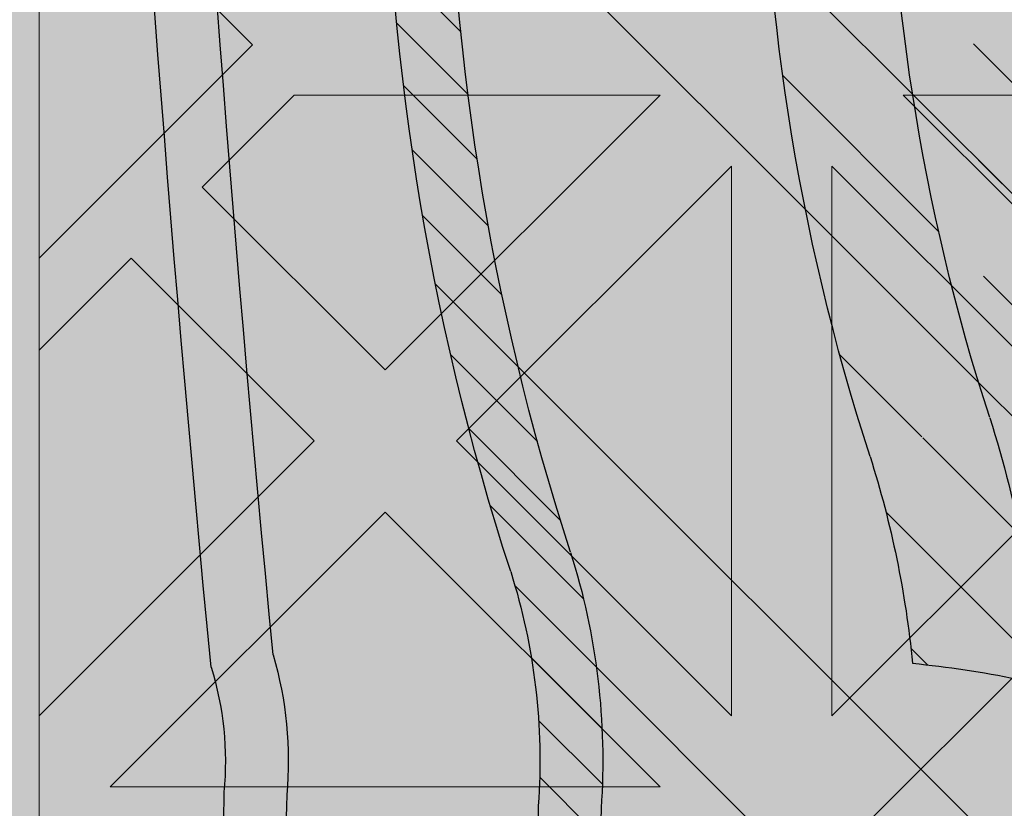
# Model space of a CAD drawing. Units: inches. Extents: x 844 to 2234, y 346 to 1084.
# Tile 28 of 93: x 1252.862 to 1255.358, y 689.183 to 691.183. Entities that reach past the tile are written whole.
import ezdxf

# ---------------------------------------------------------------- set-up
doc = ezdxf.new("R2010")
doc.units = ezdxf.units.IN
doc.header["$MEASUREMENT"] = 0
doc.layers.add('furniture', color=8, linetype='Continuous', lineweight=18)
doc.layers.add('RA-AP-01$0$INT', color=35, linetype='Continuous', lineweight=5)
doc.layers.add('RA-AP-01$0$FURN', color=3, linetype='Continuous')
doc.layers.add('RA-AP-01$0$WOOD', color=64, linetype='Continuous')

# ---------------------------------------------------------------- blocks, each defined once
blk = doc.blocks.new('A$C18D01794')
at = {"layer": 'RA-AP-01$0$INT'}
blk.add_hatch(color=256, dxfattribs=at).paths.add_polyline_path([(4.505206456958071, -6.306712009588038), (5.305206456958072, -6.306712009588038), (5.305206456958072, -7.106712009588038), (5.255206456951893, -7.10671200958804), (5.25520645694868, -6.356712009605972), (4.555206456959269, -6.356712009587461), (4.555206456956052, -7.106712009588038), (4.505206456958073, -7.106712009588038)])
h = blk.add_hatch(color=256, dxfattribs=at)
h.paths.add_polyline_path([(4.585917135068449, -6.356712009588271), (4.555206456959269, -6.35671200958746), (4.555206456959137, -6.387422687716308), (4.874495778835233, -6.706712009592356), (4.90520645695423, -6.676001331474049)])
h.paths.add_polyline_path([(5.255206456948813, -6.387422687716306), (5.255206456948682, -6.356712009605972), (5.224495778822613, -6.356712009605161), (4.905206456953498, -6.676001331474273), (4.935917135072151, -6.706712009592924)])
h.paths.add_polyline_path([(4.935917135072559, -6.706712009592068), (4.905206456953564, -6.737422687710376), (5.255206456951813, -7.087422687708613), (5.255206456951549, -7.026001331471008)])
h.paths.add_polyline_path([(4.555206456956399, -7.026001331471013), (4.555206456956134, -7.087422687708616), (4.905206456953821, -6.737422687710943), (4.874495778835166, -6.70671200959229)])
h = blk.add_hatch(color=256, dxfattribs=at)
h.paths.add_polyline_path([(4.585917135068448, -6.356712009588273), (4.614201406330596, -6.356712009589021), (4.668846067270487, -6.411356670531338), (4.723490728212344, -6.356712009591912), (4.771774999457151, -6.35671200959319), (4.826419660396886, -6.411356670535356), (4.862780050090322, -6.374996280843536), (4.844495778842715, -6.356712009595112), (4.862780050090411, -6.356712009595595), (4.905206456960182, -6.399138416468211), (4.947632863832445, -6.356712009597838), (4.965917135079675, -6.356712009598322), (4.947632863831759, -6.374996280845421), (4.983993253523576, -6.411356670538857), (5.038637914464627, -6.356712009600247), (5.08692218571208, -6.356712009601523), (5.141566846649976, -6.411356670541852), (5.196211507589851, -6.356712009604411), (5.224495778822615, -6.356712009605161), (4.905206456953975, -6.676001331473793)])
h.paths.add_polyline_path([(4.895206456956031, -6.637717060225675), (4.895206456958921, -6.528427738347902), (4.840561796018589, -6.583072399285802)], flags=16)
h.paths.add_polyline_path([(4.915206456955638, -6.637717060226121), (4.969851117895509, -6.583072399288678), (4.915206456957609, -6.528427738348344)], flags=16)
h.paths.add_polyline_path([(4.826419660395175, -6.568930263661755), (4.881064321335613, -6.514285602723745), (4.771774999456703, -6.514285602720857)], flags=16)
h.paths.add_polyline_path([(4.983993253519558, -6.568930263665262), (5.038637914460456, -6.514285602726792), (4.929348592581548, -6.514285602724816)], flags=16)
h.paths.add_polyline_path([(4.881064321336025, -6.494285602723742), (4.826419660397532, -6.439640941782821), (4.771774999457062, -6.494285602720859)], flags=16)
h.paths.add_polyline_path([(4.929348592582019, -6.494285602724817), (5.038637914460982, -6.494285602726792), (4.983993253522945, -6.439640941786327)], flags=16)
h.paths.add_polyline_path([(4.895206456960191, -6.480143467100443), (4.895206456962115, -6.407422687715913), (4.876922185715016, -6.389138416467584), (4.840561796021581, -6.425498806159401)], flags=16)
h.paths.add_polyline_path([(4.915206456958487, -6.480143467100889), (4.969851117899527, -6.425498806162279), (4.933490728206909, -6.389138416468043), (4.9152064569598, -6.40742268771434)], flags=16)
h.paths.add_polyline_path([(4.757632863832376, -6.480143467096812), (4.812277524772842, -6.425498806158772), (4.757632863834348, -6.370854145217844)], flags=16)
h.paths.add_polyline_path([(4.737632863832376, -6.480143467096286), (4.737632863834348, -6.370854145217375), (4.682988202893906, -6.425498806155385)], flags=16)
h.paths.add_polyline_path([(5.05278005008503, -6.480143467103376), (5.052780050087917, -6.370854145224413), (4.998135389146995, -6.425498806162908)], flags=16)
h.paths.add_polyline_path([(5.072780050085024, -6.480143467103744), (5.127424711025931, -6.42549880616527), (5.072780050087916, -6.370854145224832)], flags=16)
h.paths.add_polyline_path([(4.935917135072783, -6.706712009592292), (5.255206456948811, -6.387422687716309), (5.255206456948932, -6.415706958964177), (5.200561796010279, -6.470351619902839), (5.255206456949403, -6.524996280841948), (5.25520645694961, -6.5732805520894), (5.200561796009787, -6.627925213029239), (5.236922185702417, -6.664285602721864), (5.255206456949919, -6.646001331474357), (5.255206456949998, -6.664285602721898), (5.212780050078687, -6.706712009592262), (5.25520645695036, -6.749138416463932), (5.255206456950438, -6.767422687711313), (5.236922185702424, -6.749138416463297), (5.200561796009796, -6.785498806155928), (5.255206456950753, -6.840143467096874), (5.25520645695096, -6.888427738341682), (5.200561796010322, -6.943072399282328), (5.255206456951428, -6.997717060223427), (5.255206456951547, -7.026001331471006)])
h.paths.add_polyline_path([(5.042988202883395, -6.785498806155427), (5.097632863823085, -6.840143467095101), (5.097632863822622, -6.730854145216193)], flags=16)
h.paths.add_polyline_path([(5.028846067259663, -6.771356670531693), (5.083490728198774, -6.716712009592573), (4.974201406321001, -6.716712009593042)], flags=16)
h.paths.add_polyline_path([(5.117632863823087, -6.840143467095186), (5.172277524762331, -6.785498806155926), (5.11763286382262, -6.730854145216225)], flags=16)
h.paths.add_polyline_path([(5.08349072819877, -6.696712009593886), (5.028846067259652, -6.642067348654775), (4.974201406320998, -6.696712009593438)], flags=16)
h.paths.add_polyline_path([(5.131774999446817, -6.854285602718917), (5.186419660386065, -6.799640941779662), (5.241064321325782, -6.854285602719365)], flags=17)
h.paths.add_polyline_path([(5.131774999446228, -6.716712009592374), (5.186419660386065, -6.771356670532194), (5.222780050079488, -6.734996280838764), (5.204495778832781, -6.716712009592063)], flags=16)
h.paths.add_polyline_path([(5.097632863822613, -6.682569873970264), (5.097632863823061, -6.573280552091354), (5.042988202883383, -6.627925213031044)], flags=16)
h.paths.add_polyline_path([(5.131774999446899, -6.874285602718915), (5.241064321325809, -6.874285602719364), (5.186419660386591, -6.928930263658598)], flags=17)
h.paths.add_polyline_path([(5.131774999446226, -6.696712009594078), (5.204495778830767, -6.696712009594374), (5.22278005007868, -6.67842773834687), (5.186419660386049, -6.642067348654249)], flags=16)
h.paths.add_polyline_path([(5.11763286382262, -6.682569873970225), (5.17227752476232, -6.627925213030515), (5.117632863823064, -6.573280552091267)], flags=16)
h.paths.add_polyline_path([(5.186419660386069, -6.613783077405491), (5.241064321325754, -6.559138416465795), (5.131774999446791, -6.559138416466263)], flags=16)
h.paths.add_polyline_path([(5.131774999446872, -6.539138416466263), (5.24106432132578, -6.539138416465794), (5.186419660386554, -6.484493755526573)], flags=16)
h.paths.add_polyline_path([(5.255206456951811, -7.08742268770861), (5.255206456951895, -7.106712009588038), (4.555206456956052, -7.106712009588038), (4.555206456956136, -7.087422687708617), (4.905206456953973, -6.737422687710788)])
h.paths.add_polyline_path([(4.983993253513404, -6.8444937555241), (4.92934859257295, -6.899138416462108), (5.03863791445186, -6.899138416465014)], flags=16)
h.paths.add_polyline_path([(4.969851117889988, -6.83035161990006), (4.915206456952556, -6.775706958960171), (4.915206456949648, -6.884996280837944)], flags=16)
h.paths.add_polyline_path([(4.929348592572535, -6.919138416462105), (4.983993253511019, -6.973783077403037), (5.038637914451496, -6.919138416465012)], flags=16)
h.paths.add_polyline_path([(5.052780050074912, -6.93328055208906), (4.998135389134438, -6.987925213027088), (5.052780050072919, -7.042569873968025)], flags=16)
h.paths.add_polyline_path([(5.07278005007491, -6.933280552089588), (5.072780050072918, -7.042569873968497), (5.127424711013374, -6.987925213030498)], flags=16)
h.paths.add_polyline_path([(4.89520645695295, -6.775706958959721), (4.840561796013067, -6.830351619897157), (4.895206456950961, -6.884996280837494)], flags=16)
h.paths.add_polyline_path([(4.915206456948365, -6.933280552085403), (4.915206456946434, -7.006001331471951), (4.933490728192729, -7.024285602719066), (4.969851117886972, -6.987925213026453)], flags=16)
h.paths.add_polyline_path([(4.881064321327021, -6.899138416461022), (4.82641966038902, -6.84449375552057), (4.771774999448108, -6.899138416459029)], flags=16)
h.paths.add_polyline_path([(4.895206456950073, -6.933280552084951), (4.840561796009022, -6.987925213023558), (4.876922185700835, -7.024285602716997), (4.895206456948749, -7.006001331469487)], flags=16)
h.paths.add_polyline_path([(4.983993253510392, -7.0020673486505), (4.947632863816944, -7.038427738342319), (4.965917135064043, -7.05671200959023), (5.038637914448995, -7.056712009591555)], flags=16)
h.paths.add_polyline_path([(4.881064321326543, -6.91913841646102), (4.771774999447578, -6.919138416459031), (4.826419660385607, -6.973783077399508)], flags=16)
h.paths.add_polyline_path([(4.905206456946447, -7.014285602717636), (4.862780050074785, -7.056712009588352), (4.947632863816685, -7.056712009589775)], flags=16)
h.paths.add_polyline_path([(5.14156684663679, -7.002067348654549), (5.086922185696452, -7.056712009592438), (5.196211507574223, -7.056712009594425)], flags=16)
h.paths.add_polyline_path([(4.8264196603837, -7.002067348646972), (4.771774999442643, -7.056712009585575), (4.8444957788276, -7.056712009587508), (4.862780050075511, -7.038427738340416)], flags=16)
h.paths.add_polyline_path([(4.812277524760289, -6.98792521302292), (4.757632863822258, -6.933280552082447), (4.757632863819352, -7.042569873961408)], flags=16)
h.paths.add_polyline_path([(4.73763286382226, -6.933280552082079), (4.682988202881349, -6.987925213020536), (4.737632863819352, -7.04256987396099)], flags=16)
h.paths.add_polyline_path([(4.723490728195188, -7.056712009584289), (4.668846067257299, -7.002067348643949), (4.614201406317417, -7.056712009581383)], flags=16)
h.paths.add_polyline_path([(4.597632863829262, -6.706712009592262), (4.555206456957951, -6.664285602721896), (4.555206456958029, -6.646001331474357), (4.573490728205535, -6.664285602721864), (4.609851117898167, -6.627925213029238), (4.555206456958338, -6.573280552089402), (4.555206456958546, -6.524996280841952), (4.60985111789767, -6.470351619902839), (4.555206456959015, -6.415706958964177), (4.555206456959138, -6.387422687716309), (4.874495778835167, -6.70671200959229), (4.5552064569564, -7.026001331471015), (4.555206456956523, -6.997717060223433), (4.609851117897629, -6.94307239928233), (4.555206456956988, -6.888427738341681), (4.555206456957198, -6.840143467096881), (4.609851117898153, -6.78549880615593), (4.573490728205528, -6.749138416463297), (4.555206456957507, -6.76742268771132), (4.555206456957585, -6.749138416463933)])
h.paths.add_polyline_path([(4.712780050085332, -6.730854145216195), (4.712780050084863, -6.840143467095105), (4.767424711024555, -6.785498806155427)], flags=16)
h.paths.add_polyline_path([(4.726922185709173, -6.716712009592573), (4.781566846648288, -6.771356670531693), (4.836211507586949, -6.716712009593043)], flags=16)
h.paths.add_polyline_path([(4.692780050085327, -6.730854145216225), (4.638135389145619, -6.785498806155928), (4.692780050084865, -6.840143467095185)], flags=16)
h.paths.add_polyline_path([(4.726922185709182, -6.696712009593886), (4.836211507586949, -6.696712009593436), (4.7815668466483, -6.642067348654773)], flags=16)
h.paths.add_polyline_path([(4.678637914461726, -6.71671200959237), (4.605917135075169, -6.716712009592063), (4.587632863828464, -6.734996280838766), (4.623993253521887, -6.771356670532195)], flags=16)
h.paths.add_polyline_path([(4.712780050085336, -6.68256987397026), (4.767424711024568, -6.627925213031042), (4.71278005008489, -6.573280552091352)], flags=16)
h.paths.add_polyline_path([(4.678637914461726, -6.696712009594076), (4.623993253521899, -6.642067348654247), (4.587632863829271, -6.67842773834687), (4.605917135077185, -6.696712009594376)], flags=16)
h.paths.add_polyline_path([(4.692780050085336, -6.682569873970228), (4.692780050084889, -6.573280552091267), (4.638135389145632, -6.627925213030515)], flags=16)
h.paths.add_polyline_path([(4.623993253521885, -6.799640941779662), (4.678637914461131, -6.854285602718915), (4.56934859258217, -6.854285602719365)], flags=17)
h.paths.add_polyline_path([(4.623993253521901, -6.613783077405509), (4.678637914461158, -6.559138416466263), (4.569348592582195, -6.559138416465795)], flags=16)
h.paths.add_polyline_path([(4.678637914461051, -6.874285602718915), (4.623993253521361, -6.928930263658598), (4.569348592582143, -6.874285602719364)], flags=17)
h.paths.add_polyline_path([(4.678637914461076, -6.539138416466263), (4.623993253521399, -6.484493755526573), (4.569348592582167, -6.539138416465796)], flags=16)
h = blk.add_hatch(color=256, dxfattribs=at)
h.paths.add_polyline_path([(5.028846067259997, -6.642067348655121), (4.974201406321342, -6.696712009593783), (5.083490728199115, -6.69671200959423)])
h.paths.add_polyline_path([(4.974201406321344, -6.716712009593388), (5.028846067260004, -6.771356670532039), (5.083490728199117, -6.716712009592919)])
h.paths.add_polyline_path([(5.042988202883738, -6.785498806155768), (5.097632863823428, -6.840143467095449), (5.097632863822963, -6.73085414521654)])
h.paths.add_polyline_path([(5.117632863822961, -6.730854145216568), (5.117632863823428, -6.840143467095531), (5.172277524762674, -6.785498806156272)])
h.paths.add_polyline_path([(5.131774999446572, -6.716712009592718), (5.186419660386406, -6.77135667053254), (5.222780050079831, -6.734996280839116), (5.204495778833122, -6.716712009592409)])
h.paths.add_polyline_path([(5.236922185702764, -6.749138416463644), (5.200561796010139, -6.785498806156274), (5.255206456949971, -6.840143467096101), (5.255206456950271, -6.76742268771115)])
h.paths.add_polyline_path([(5.186419660386412, -6.799640941780006), (5.131774999447164, -6.854285602719262), (5.241064321326123, -6.854285602719711)])
h.paths.add_polyline_path([(5.131774999447238, -6.874285602719261), (5.186419660386934, -6.928930263658944), (5.241064321326153, -6.874285602719709)])
h.paths.add_polyline_path([(5.200561796010663, -6.943072399282675), (5.255206456949324, -6.997717060221329), (5.255206456949777, -6.888427738343558)])
h.paths.add_polyline_path([(5.21278005007903, -6.706712009592607), (5.255206456950223, -6.749138416463798), (5.255206456950696, -6.664285602721891)])
h.paths.add_polyline_path([(5.13177499944657, -6.696712009594424), (5.204495778831106, -6.696712009594723), (5.222780050079024, -6.678427738347219), (5.186419660386397, -6.642067348654592)])
h.paths.add_polyline_path([(5.117632863823405, -6.573280552091611), (5.117632863822955, -6.682569873970578), (5.172277524762665, -6.627925213030859)])
h.paths.add_polyline_path([(5.042988202883727, -6.627925213031387), (5.097632863822957, -6.682569873970603), (5.097632863823407, -6.573280552091697)])
h.paths.add_polyline_path([(5.131774999447135, -6.559138416466609), (5.186419660386394, -6.613783077405857), (5.241064321326097, -6.559138416466144)])
h.paths.add_polyline_path([(5.200561796010128, -6.627925213029584), (5.236922185702758, -6.664285602722211), (5.255206456950264, -6.646001331474705), (5.255206456949948, -6.573280552089752)])
h.paths.add_polyline_path([(5.186419660386895, -6.484493755526919), (5.131774999447213, -6.539138416466609), (5.241064321326127, -6.539138416466142)])
h.paths.add_polyline_path([(5.200561796010624, -6.470351619903183), (5.255206456949745, -6.524996280842298), (5.255206456949276, -6.415706958964523)])
for p, q in [((5.255206456951895, -7.106712009588038), (5.255206456948681, -6.356712009605972)), ((4.935917135072783, -6.706712009592292), (5.255206456948813, -6.387422687716307)), ((5.131774999446792, -6.559138416466263), (5.241064321325755, -6.559138416465795)), ((5.131774999446792, -6.559138416466263), (5.186419660386049, -6.613783077405509)), ((5.241064321325755, -6.559138416465795), (5.186419660386049, -6.613783077405509)), ((5.042988202883385, -6.627925213031041), (5.097632863823062, -6.573280552091352)), ((5.097632863823062, -6.573280552091352), (5.097632863822615, -6.682569873970262)), ((5.117632863823062, -6.573280552091267), (5.172277524762319, -6.627925213030515)), ((5.117632863823062, -6.573280552091267), (5.117632863822614, -6.68256987397023)), ((5.255206456949605, -6.573280552089405), (5.200561796009783, -6.627925213029239)), ((5.255206456949918, -6.646001331474357), (5.255206456949605, -6.573280552089405)), ((5.097632863822615, -6.682569873970262), (5.042988202883383, -6.627925213031042)), ((5.117632863822614, -6.68256987397023), (5.172277524762319, -6.627925213030515)), ((5.200561796009783, -6.627925213029238), (5.236922185702415, -6.664285602721863)), ((5.083490728198769, -6.696712009593882), (5.028846067259652, -6.642067348654775)), ((5.131774999446228, -6.696712009594078), (5.186419660386053, -6.642067348654247)), ((5.186419660386051, -6.642067348654247), (5.222780050078681, -6.67842773834687)), ((5.255206456949919, -6.646001331474357), (5.236922185702415, -6.664285602721864)), ((5.212780050078687, -6.706712009592262), (5.255206456950353, -6.664285602721543)), ((5.25520645694988, -6.74913841646345), (5.255206456950353, -6.664285602721543)), ((5.204495778833082, -6.69671200959206), (5.222780050078681, -6.67842773834687)), ((5.08349072819877, -6.696712009593886), (4.974201406320999, -6.696712009593436)), ((5.204495778831179, -6.696712009594376), (5.131774999446228, -6.696712009594078)), ((5.212780050078687, -6.706712009592262), (5.25520645694988, -6.74913841646345))]:
    blk.add_line(p, q, dxfattribs=at)
blk = doc.blocks.new('A$C32926AE1')
at = {"layer": 'RA-AP-01$0$FURN'}
h = blk.add_hatch(dxfattribs=at)
h.set_pattern_fill('ANSI31', color=256, scale=0.1, style=0)
h.set_pattern_definition([(45, (0, 0), (-0.0088388347648318, 0.0088388347648318), [])])
edge = h.paths.add_edge_path(flags=16)
edge.add_arc((4.904771284329206, 4.246793130718756), 0.2603971832811541, 75.22398030683196, 104.7760196931204)
edge.add_arc((4.904771284329206, 4.246793130718756), 0.2603971832811541, 75.223980306832, 104.77601969312039, ccw=False)
edge = h.paths.add_edge_path(flags=16)
edge.add_arc((4.904771284329206, 4.067062675376612), 0.2603971832811541, 255.2239803068796, 284.776019693168)
edge.add_arc((4.904771284329206, 4.067062675376612), 0.2603971832811541, 255.22398030687958, 284.77601969316805, ccw=False)
edge = h.paths.add_edge_path(flags=0)
edge.add_arc((4.904771284329206, 4.067062675376612), 0.2603971832811541, 255.2239803068796, 284.776019693168)
edge.add_arc((4.904771284329206, 4.067062675376612), 0.2603971832811541, 255.22398030687958, 284.77601969316805, ccw=False)
edge = h.paths.add_edge_path(flags=0)
edge.add_arc((4.904771284329206, 4.067062675376612), 0.2603971832811541, 255.2239803068796, 284.776019693168)
edge.add_arc((4.904771284329206, 4.067062675376612), 0.2603971832811541, 255.22398030687958, 284.77601969316805, ccw=False)
edge = h.paths.add_edge_path()
edge.add_arc((4.604388392048174, 4.588829985554312), 0.1599999999999918, 342.3781640246255, 354.4317409793762)
edge.add_arc((5.090145208887507, 4.43216705527679), 0.3503971832811637, 162.0091218307731, 180.3186872093483)
edge.add_arc((5.205154176610243, 4.588829985554953), 0.1599999999999917, 185.5682590208461, 197.6218359767349)
edge.add_arc((4.904771284329229, 4.246793130718735), 0.3503971832811761, 72.00912183053516, 107.9908781690354)
edge.add_arc((9.535952835716557, 4.28682295566602), 4.798342501046485, 178.2875002453811, 181.5576802719453)
edge.add_arc((4.719397359771122, 4.43216705527679), 0.3503971832811637, 359.6813127906516, 377.9908781692269)
edge.add_arc((9.535967292294904, 4.286822350292874), 4.778371420254705, 178.2965938931842, 181.5667745797229)
edge.add_arc((4.719397359771122, 4.43216705527679), 0.3303971832811637, 359.6813127906516, 377.9908781692269)
edge.add_arc((0.2735752763637294, 4.286822350292874), 4.7783714202547, 358.4332254202771, 361.7034061068158)
edge.add_arc((5.061434214606998, 4.732549947558029), 0.1600000000000254, 252.3781640250584, 264.4317409792362)
edge.add_arc((4.748108354051257, 4.732549947558012), 0.1600000000000541, 275.5682590208426, 287.6218359759532)
edge.add_arc((4.604388392048115, 4.588829985554317), 0.1800000000000505, 342.3567572500182, 349.3735009646207)
edge.add_arc((5.205154176610254, 4.588829985554976), 0.1800000000000069, 190.6264990356027, 197.6432427513933)
edge.add_arc((5.061434214607106, 4.732549947558013), 0.1800000000000424, 252.3567572496606, 259.3735009644582)
edge.add_arc((4.904771284329208, 4.246793130718737), 0.3303971832811676, 71.99844483668534, 108.0015551637021)
edge.add_arc((4.748108354051414, 4.732549947558045), 0.1800000000000547, 280.6264990355479, 287.6432427495938)
edge.add_arc((5.090145208887514, 4.432167055276789), 0.2803971832811691, 162.8706300666893, 180.816523289902)
edge.add_arc((4.719397359771136, 4.432167055276689), 0.2803971832811534, 359.183476710103, 377.1293699333214)
edge.add_arc((4.904771284329222, 4.246793130718737), 0.2803971832811769, 72.87063006672916, 107.1293699332334)
edge.add_arc((5.090145208887522, 4.432167055276788), 0.2603971832811776, 165.2239803068007, 180.9953123810312)
edge.add_arc((4.719397359771141, 4.432167055276699), 0.2603971832811458, 359.0046876189768, 374.7760196932087)
edge.add_arc((5.090145208887507, 4.43216705527679), 0.3303971832811637, 162.0091218307731, 180.3186872093483)
edge.add_arc((9.53595427642584, 4.285015535491528), 4.728345371032053, 178.265043920078, 181.5679956281801)
edge.add_arc((0.2735882922327999, 4.285015535491582), 4.728345371032045, 358.4320043718193, 361.7349560799204)
edge.add_arc((9.535953591267507, 4.284458026472751), 4.708343996644348, 178.2573054306777, 181.5704995759608)
edge.add_arc((0.273588977391114, 4.284458026472785), 4.708343996644358, 358.4295004240388, 361.7426945693213)
edge.add_arc((0.2735889773911131, 4.029397779622582), 4.708343996644359, 358.2573054306787, 361.5704995759613)
edge.add_arc((9.535953591267518, 4.029397779622618), 4.708343996644359, 178.4295004240391, 181.7426945693223)
edge.add_arc((0.2735882922327901, 4.028840270603786), 4.728345371032054, 358.2650439200796, 361.5679956281808)
edge.add_arc((9.53595427642584, 4.028840270603841), 4.728345371032054, 178.4320043718199, 181.7349560799219)
edge.add_arc((0.2735752763637302, 4.027033455802493), 4.778371420254699, 358.2965938931842, 361.5667745797229)
edge.add_arc((4.719397359771122, 3.881688750818578), 0.3303971832811637, 342.0091218307731, 360.3186872093484)
edge.add_arc((5.090145208887507, 3.881688750818578), 0.3303971832811637, 179.6813127906516, 197.9908781692269)
edge.add_arc((9.535967292294904, 4.027033455802493), 4.778371420254705, 178.433225420277, 181.7034061068158)
edge.add_arc((4.719397359771122, 3.881688750818578), 0.3503971832811637, 342.0091218307731, 360.3186872093484)
edge.add_arc((9.53595283571655, 4.027032850429349), 4.79834250104648, 178.4423197280546, 181.7124997546188)
edge.add_arc((4.719397359771141, 3.881688750818669), 0.2603971832811458, 345.2239803067913, 360.9953123810232)
edge.add_arc((5.090145208887522, 3.88168875081858), 0.2603971832811776, 179.0046876189687, 194.7760196931993)
edge.add_arc((4.904771284329222, 4.067062675376631), 0.2803971832811769, 252.8706300667665, 287.1293699332708)
edge.add_arc((4.719397359771136, 3.881688750818678), 0.2803971832811534, 342.8706300666787, 360.8165232898969)
edge.add_arc((5.090145208887514, 3.881688750818579), 0.2803971832811691, 179.183476710098, 197.1293699333106)
edge.add_arc((4.748108354051414, 3.581305858537323), 0.1800000000000547, 72.3567572504062, 79.37350096445199)
edge.add_arc((4.904771284329208, 4.067062675376631), 0.3303971832811676, 251.9984448362979, 288.0015551633146)
edge.add_arc((5.061434214607106, 3.581305858537355), 0.1800000000000424, 100.6264990355418, 107.6432427503394)
edge.add_arc((5.205154176610254, 3.725025820540392), 0.1800000000000069, 162.3567572486066, 169.3735009643972)
edge.add_arc((4.604388392048115, 3.725025820541051), 0.1800000000000505, 10.62649903537925, 17.64324274998182)
edge.add_arc((4.748108354051257, 3.581305858537356), 0.1600000000000541, 72.37816402404681, 84.43174097915735)
edge.add_arc((4.904771284329229, 4.067062675376632), 0.3503971832811761, 252.0091218309645, 287.9908781694648)
edge.add_arc((5.061434214606998, 3.581305858537339), 0.1600000000000254, 95.56825902076373, 107.6218359749416)
edge.add_arc((5.205154176610243, 3.725025820540414), 0.1599999999999917, 162.3781640232651, 174.4317409791539)
edge.add_arc((5.090145208887507, 3.881688750818578), 0.3503971832811637, 179.6813127906516, 197.9908781692269)
edge.add_arc((4.604388392048174, 3.725025820541056), 0.1599999999999918, 5.568259020623824, 17.62183597537444)
edge.add_arc((0.2735897329420762, 4.28682295566602), 4.798342501046482, 358.4423197280547, 361.7124997546188)
edge.add_arc((0.2735897329420691, 4.027032850429348), 4.798342501046489, 358.2875002453812, 361.5576802719453)
at = {"layer": 'RA-AP-01$0$WOOD'}
h = blk.add_hatch(color=256, dxfattribs=at)
h.dxf.hatch_style = 1
h.paths.add_polyline_path([(5.157430609644524, 4.573483066760929, -0.1009492694046607), (5.155401577623758, 4.593365984175333, -0.1842662638101597), (5.172249623284174, 4.638795604568598, 0.2056608120311276), (5.179560981299304, 4.661316324430096, 0.3614336704623542), (5.134352340494423, 4.706524965234944, 0.2056608120311297), (5.111831620632933, 4.699213607219793, -0.1842662638101113), (5.066402000239693, 4.682365561559342, -0.1055311479399994), (5.045656153913092, 4.68467289944697, 0.1567636581983829), (4.763886414745334, 4.684672899446966, -0.1055311479399895), (4.743140568418733, 4.68236556155934, -0.1842662638100833), (4.6977109480255, 4.69921360721979, 0.2056608120302612), (4.675190228164109, 4.706524965234949, 0.3614336704708441), (4.629981587358889, 4.66131632442871, 0.2056608120245944), (4.637292945374126, 4.638795604567974, -0.1842662638101024), (4.654140991034615, 4.59336598417475, -0.1009492694055169), (4.652111959013835, 4.573483066760181, 0.021410119221476), (4.629748025606143, 4.156712009541676, 0.0214101192214795), (4.652111959013809, 3.739940952323101, -0.1009492694059586), (4.654140991034615, 3.720058034908448, -0.1842662638100975), (4.637292945374126, 3.674628414515226, 0.2056608120245705), (4.629981587358889, 3.652107694654492, 0.3614336704708879), (4.675190228164113, 3.606899053848249, 0.2056608120302384), (4.697710948025501, 3.614210411863408, -0.1842662638100995), (4.743140568418738, 3.63105845752386, -0.1055311479402541), (4.763886414745388, 3.628751119636215, 0.1567636581983776), (5.045656153913137, 3.628751119636244, -0.1055311479397538), (5.066402000239692, 3.631058457523857, -0.1842662638101067), (5.111831620632931, 3.614210411863407, 0.2056608120310924), (5.134352340494417, 3.606899053848256, 0.3614336704624001), (5.179560981299307, 3.652107694653103, 0.2056608120311314), (5.172249623284175, 3.6746284145146, -0.1842662638101402), (5.155401577623758, 3.72005803490786, -0.1009492694051366), (5.15743060964455, 3.739940952322354, 0.0214101192215073), (5.179794543052287, 4.156712009541468, 0.0214101192215252)])
h.paths.add_polyline_path([(4.639748609479751, 4.156712009541513, 0.0213537860821624), (4.661970494867118, 3.741887061152232, -0.094075836301374), (4.664143710413708, 3.7196126951003, -0.1824818158568985), (4.644813765429836, 3.668037719127816, 0.2056608120245319), (4.639939526753007, 3.653023905887301, 0.3614336704710246), (4.676106439397173, 3.616856993242342, 0.2056608120302234), (4.691120252638095, 3.621731231919122, -0.1824818158602558), (4.742695228611606, 3.641061176902986, -0.1029891339458722), (4.766991894714349, 3.638256818950944, 0.156709409989566), (5.042550673941472, 3.638256818950105, -0.102989133958497), (5.066847340047078, 3.641061176902949, -0.1824818158594995), (5.118422316020358, 3.621731231919103, 0.2056608120311416), (5.133436129261316, 3.616856993242346, 0.3614336704621468), (5.169603041905217, 3.653023905886178, 0.2056608120310986), (5.164728803228477, 3.668037719127177, -0.1824818158565612), (5.145398858244737, 3.719612695099578, -0.0940758363009313), (5.147572073791232, 3.741887061151398, 0.0213537860822023), (5.169793959178681, 4.156712009541451, 0.0213537860822226), (5.147572073791203, 4.571536957931898, -0.0940758363005034), (5.145398858244737, 4.59381132398362, -0.1824818158565587), (5.164728803228476, 4.645386299956021, 0.2056608120311045), (5.169603041905216, 4.66040011319702, 0.3614336704621845), (5.133436129261313, 4.696567025840856, 0.2056608120310773), (5.118422316020359, 4.691692787164098, -0.182481815859508), (5.066847340047078, 4.67236284218025, -0.1029891339584606), (5.04255067394148, 4.675167200133092, 0.156709409989566), (4.766991894714357, 4.675167200132257, -0.1029891339458842), (4.742695228611611, 4.672362842180213, -0.1824818158602725), (4.691120252638095, 4.691692787164077, 0.2056608120302152), (4.676106439397174, 4.696567025840858, 0.3614336704710363), (4.639939526753005, 4.660400113195899, 0.2056608120245495), (4.644813765429837, 4.645386299955384, -0.1824818158568934), (4.664143710413708, 4.593811323982902, -0.0940758363009187), (4.661970494867149, 4.571536957931074, 0.021353786082177)], flags=16)
h.paths.add_polyline_path([(5.129794543052235, 4.432167055276933, -0.0141661062790638), (5.130152669293814, 4.156927903047693, -0.0141661062790647), (5.129794543052234, 3.881688750818433, -0.0785247771143638), (5.10979738006795, 3.755143611847103, 0.0945969212073497), (5.105408519571111, 3.717898134952927, 0.1043170707844957), (5.116074640131521, 3.670385395016088, 0.1043170707864965), (5.068561900193738, 3.681051515576561, 0.09459692119553), (5.031316423304057, 3.676662655080835, -0.1580239521427272), (4.778226145355827, 3.676662655080367, 0.0945969211986668), (4.740980668464973, 3.681051515576592, 0.1043170707882822), (4.693467928526415, 3.670385395015844, 0.1043170707867916), (4.704134049087309, 3.717898134953662, 0.0945969211972894), (4.69974518859162, 3.755143611844042, -0.0785247771163196), (4.679748025606343, 3.881688750818406, -0.0141661062790663), (4.679389899364763, 4.156927903047693, -0.0141661062790672), (4.679748025606343, 4.432167055276998, -0.0785247771163064), (4.699745188591625, 4.55871219425134, 0.094596921197333), (4.704134049087308, 4.595957671141738, 0.1043170707867205), (4.693467928526416, 4.643470411079523, 0.1043170707882628), (4.740980668464965, 4.632804290518776, 0.0945969211988114), (4.778226145355874, 4.637193151015016, -0.158023952142669), (5.031316423304015, 4.637193151014546, 0.0945969211956361), (5.068561900193736, 4.632804290518806, 0.1043170707864979), (5.11607464013152, 4.643470411079278, 0.1043170707844617), (5.105408519571112, 4.595957671142455, 0.0945969212074597), (5.109797380067959, 4.558712194248236, -0.0785247771143467)], flags=0)
h.paths.add_polyline_path([(5.119794532311105, 4.432259799204851, -0.0142000800617244), (5.120156169157484, 4.156927903047701, -0.0142000800617277), (5.119794532311105, 3.881596006890482, -0.0784894509520253), (5.100273383573699, 3.758192358677797, 0.0940138827242913), (5.095413455884425, 3.717477693979438, 0.0606271852308753), (5.099615656341024, 3.686844378806616, 0.0606271852322524), (5.068982341167493, 3.691046579263239, 0.0940138827010453), (5.028267676478798, 3.686186651576848, -0.1580706864508061), (4.781274892180912, 3.686186651576435, 0.0940138827026903), (4.740560227491556, 3.691046579263279, 0.0606271852339895), (4.709926912317155, 3.686844378806508, 0.0606271852329405), (4.714129112773991, 3.717477693980356, 0.094013882701304), (4.709269185087677, 3.758192358669163, -0.0784894509577193), (4.689748036347473, 3.881596006890469, -0.014200080061729), (4.689386399501094, 4.156927903047709, -0.0142000800617217), (4.689748036347473, 4.432259799204808, -0.078489450957724), (4.709269185087651, 4.555663447426125, 0.0940138827014585), (4.714129112773992, 4.596378112114996, 0.0606271852329731), (4.709926912317154, 4.62701142728886, 0.0606271852340196), (4.74056022749157, 4.622809226832087, 0.0940138827024997), (4.781274892180847, 4.627669154518912, -0.1580706864508359), (5.028267676478777, 4.627669154518526, 0.0940138827010946), (5.068982341167492, 4.622809226832129, 0.060627185232254), (5.099615656341024, 4.627011427288751, 0.0606271852308727), (5.095413455884425, 4.59637811211593, 0.0940138827241088), (5.100273383573675, 4.555663447417647, -0.0784894509520978)], flags=0)
h.paths.add_polyline_path([(5.06978912287499, 4.430218106756144, -0.014241683694547), (5.070173729147532, 4.156927903047672, -0.0142416836945458), (5.06978912287499, 3.883637699339223, -0.0800609523125196), (5.052662118612511, 3.773463122773442, 0.0526421978001116), (5.04590916754064, 3.740550867606997, 0.0526421977992423), (5.012996912374707, 3.73379791653534, -0.1583028414718258), (4.796545656286308, 3.73379791653451, 0.0526421978034211), (4.763633401117837, 3.740550867607021, 0.0526421978018622), (4.756880450045755, 3.773463122774558, -0.0800609523117106), (4.739753445783639, 3.883637699339268, -0.0142416836945435), (4.739368839511098, 4.156927903047671, -0.0142416836945477), (4.739753445783639, 4.430218106756155, -0.0800609523116345), (4.75688045004574, 4.540392683320762, 0.052642197801941), (4.763633401117837, 4.573304938488346, 0.0526421978035071), (4.796545656286361, 4.580057889560873, -0.1583028414717561), (5.012996912374669, 4.580057889560039, 0.0526421977993048), (5.04590916754064, 4.57330493848837, 0.0526421978002057), (5.052662118612529, 4.540392683321868, -0.080060952312477)], flags=0)
h.paths.add_polyline_path([(5.049789715110557, 4.43038092723357, -0.0143097550741839), (5.05018085590259, 4.156927903047715, -0.0143097550741854), (5.049789715110558, 3.883474878861827, -0.0800685599149176), (5.03362098255317, 3.779581877367999, 0.0306258898956367), (5.028241146483733, 3.758218888663947, 0.0306258898977031), (5.006878157778253, 3.75283905259408, -0.1583983521624096), (4.802664410878162, 3.752839052594731, 0.0306258898946014), (4.781301422174808, 3.758218888663924, 0.0306258898967912), (4.775921586105202, 3.779581877368794, -0.080068559914251), (4.759752853548071, 3.883474878861786, -0.0143097550741854), (4.759361712756037, 4.156927903047671, -0.0143097550741854), (4.759752853548071, 4.430380927233557, -0.0800685599142479), (4.775921586105193, 4.534273928726546, 0.0306258898968306), (4.781301422174808, 4.555636917431444, 0.0306258898945754), (4.802664410878143, 4.561016753500631, -0.1583983521624168), (5.006878157778244, 4.561016753501291, 0.0306258898977177), (5.028241146483733, 4.555636917431421, 0.0306258898958182), (5.03362098255321, 4.534273928727244, -0.080068559914796)], flags=0)
h.paths.add_polyline_path([(4.999766070382627, 4.428171244713864, -0.0143443147609634), (5.000198441819402, 4.156927903047689, -0.0143443147609612), (4.999766070382627, 3.885684561381556, -0.0784641635803329), (4.987356730658798, 3.799103304488872, -0.1506053783831347), (4.822185837999821, 3.79910330448882, -0.0784641635803318), (4.809776498276007, 3.885684561381509, -0.014344314760963), (4.809344126839227, 4.156927903047677, -0.0143443147609645), (4.809776498276007, 4.428171244713873, -0.0784641635803192), (4.822185837999822, 4.514752501606549, -0.1506053783831338), (4.987356730658798, 4.514752501606494, -0.078464163580285)], flags=0)
h.paths.add_polyline_path([(4.979755254238824, 4.42764379880488, -0.0143772539198268), (4.980205517789977, 4.156927903047693, -0.0143772539198275), (4.979755254238824, 3.886212007290489, -0.0689242507424422), (4.971183264704897, 3.815276770442801, -0.1296645318904179), (4.838359303953726, 3.815276770442746, -0.0689242507424186), (4.829787314419809, 3.886212007290419, -0.0143772539198292), (4.829337050868653, 4.156927903047653, -0.0143772539198325), (4.829787314419809, 4.427643798804946, -0.0689242507424211), (4.838359303953725, 4.498579035652621, -0.1296645318904187), (4.971183264704897, 4.498579035652565, -0.0689242507424401)], flags=0)
h = blk.add_hatch(color=256, dxfattribs=at)
h.dxf.hatch_style = 1
h.paths.add_polyline_path([(5.145398858244737, 4.59381132398362, -0.1824818158565616), (5.164728803228476, 4.645386299956021, 0.2056608120311045), (5.169603041905216, 4.66040011319702, 0.3614336704621845), (5.133436129261313, 4.696567025840856, 0.2056608120310773), (5.118422316020359, 4.691692787164098, -0.182481815859508), (5.066847340047078, 4.67236284218025, -0.1029891339584606), (5.04255067394148, 4.675167200133092, 0.156709409989566), (4.766991894714357, 4.675167200132257, -0.1029891339458842), (4.742695228611611, 4.672362842180213, -0.1824818158602725), (4.691120252638095, 4.691692787164077, 0.2056608120302152), (4.676106439397174, 4.696567025840858, 0.3614336704710363), (4.639939526753005, 4.660400113195899, 0.2056608120245495), (4.644813765429837, 4.645386299955384, -0.1824818158568934), (4.664143710413708, 4.593811323982902, -0.0940758363009187), (4.661970494867149, 4.571536957931074, 0.0213537860821772), (4.639748609479751, 4.156712009541507, 0.0213537860821625), (4.661970494867119, 3.741887061152226, -0.0940758363013071), (4.664143710413708, 3.719612695100309, -0.1824818158569294), (4.644813765429836, 3.668037719127816, 0.2056608120245319), (4.639939526753007, 3.653023905887301, 0.3614336704710246), (4.676106439397173, 3.616856993242342, 0.2056608120302234), (4.691120252638095, 3.621731231919122, -0.1824818158602558), (4.742695228611606, 3.641061176902986, -0.1029891339458722), (4.766991894714349, 3.638256818950944, 0.156709409989566), (5.042550673941472, 3.638256818950105, -0.102989133958497), (5.066847340047078, 3.641061176902949, -0.1824818158594995), (5.118422316020358, 3.621731231919103, 0.2056608120311416), (5.133436129261316, 3.616856993242346, 0.3614336704621468), (5.169603041905217, 3.653023905886178, 0.2056608120310986), (5.164728803228477, 3.668037719127177, -0.1824818158565612), (5.145398858244737, 3.719612695099578, -0.0940758363009313), (5.147572073791232, 3.741887061151398, 0.0213537860822023), (5.169793959178681, 4.156712009541451, 0.0213537860822226), (5.147572073791203, 4.571536957931898, -0.0940758363004996)])
h.paths.add_polyline_path([(5.109797380067958, 4.55871219424824, -0.0785247771143472), (5.129794543052234, 4.432167055276936, -0.0141661062790644), (5.130152669293814, 4.156927903047685, -0.014166106279066), (5.129794543052234, 3.881688750818401, -0.0785247771143517), (5.109797380067946, 3.755143611847092, 0.0945969212073132), (5.105408519571111, 3.717898134952929, 0.1043170707844995), (5.116074640131521, 3.670385395016088, 0.1043170707864965), (5.068561900193738, 3.681051515576561, 0.09459692119553), (5.031316423304057, 3.676662655080835, -0.1580239521427272), (4.778226145355827, 3.676662655080367, 0.0945969211986668), (4.740980668464973, 3.681051515576592, 0.1043170707882822), (4.693467928526415, 3.670385395015844, 0.1043170707867916), (4.704134049087309, 3.717898134953662, 0.0945969211972894), (4.69974518859162, 3.755143611844042, -0.0785247771163196), (4.679748025606343, 3.881688750818406, -0.0141661062790663), (4.679389899364763, 4.156927903047693, -0.0141661062790672), (4.679748025606343, 4.432167055276998, -0.0785247771163064), (4.699745188591625, 4.55871219425134, 0.094596921197333), (4.704134049087308, 4.595957671141738, 0.1043170707867205), (4.693467928526416, 4.643470411079523, 0.1043170707882628), (4.740980668464965, 4.632804290518776, 0.0945969211988114), (4.778226145355874, 4.637193151015016, -0.158023952142669), (5.031316423304015, 4.637193151014546, 0.0945969211956361), (5.068561900193736, 4.632804290518806, 0.1043170707864979), (5.11607464013152, 4.643470411079278, 0.1043170707844617), (5.105408519571112, 4.595957671142455, 0.0945969212074504)], flags=16)
h.paths.add_polyline_path([(5.100273383573655, 4.55566344741771, -0.0784894509521388), (5.119794532311105, 4.432259799204852, -0.0142000800617252), (5.120156169157484, 4.156927903047686, -0.014200080061726), (5.119794532311105, 3.881596006890502, -0.0784894509520446), (5.100273383573696, 3.758192358677786, 0.0940138827242721), (5.095413455884425, 3.717477693979436, 0.0606271852308692), (5.099615656341024, 3.686844378806616, 0.0606271852322522), (5.068982341167493, 3.691046579263239, 0.0940138827010453), (5.028267676478798, 3.686186651576848, -0.1580706864508061), (4.781274892180912, 3.686186651576435, 0.0940138827026903), (4.740560227491556, 3.691046579263279, 0.0606271852339895), (4.709926912317155, 3.686844378806508, 0.0606271852329405), (4.714129112773991, 3.717477693980356, 0.094013882701304), (4.709269185087677, 3.758192358669163, -0.0784894509577193), (4.689748036347473, 3.881596006890469, -0.014200080061729), (4.689386399501094, 4.156927903047709, -0.0142000800617217), (4.689748036347473, 4.432259799204808, -0.078489450957724), (4.709269185087651, 4.555663447426125, 0.0940138827014585), (4.714129112773992, 4.596378112114996, 0.0606271852329731), (4.709926912317154, 4.62701142728886, 0.0606271852340196), (4.74056022749157, 4.622809226832087, 0.0940138827024997), (4.781274892180847, 4.627669154518912, -0.1580706864508359), (5.028267676478777, 4.627669154518526, 0.0940138827010946), (5.068982341167492, 4.622809226832129, 0.060627185232254), (5.099615656341024, 4.627011427288751, 0.0606271852308727), (5.095413455884425, 4.59637811211593, 0.094013882723957)], flags=0)
h.paths.add_polyline_path([(5.04590916754064, 4.57330493848837, 0.0526421978002057), (5.052662118612529, 4.540392683321868, -0.0800609523124783), (5.06978912287499, 4.430218106756142, -0.0142416836945469), (5.070173729147532, 4.156927903047672, -0.0142416836945458), (5.06978912287499, 3.883637699339223, -0.0800609523125196), (5.052662118612511, 3.773463122773442, 0.0526421978001116), (5.04590916754064, 3.740550867606997, 0.0526421977992423), (5.012996912374707, 3.73379791653534, -0.1583028414718258), (4.796545656286308, 3.73379791653451, 0.0526421978034211), (4.763633401117837, 3.740550867607021, 0.0526421978018622), (4.756880450045755, 3.773463122774558, -0.0800609523117106), (4.739753445783639, 3.883637699339268, -0.0142416836945435), (4.739368839511098, 4.156927903047671, -0.0142416836945477), (4.739753445783639, 4.430218106756155, -0.0800609523116345), (4.75688045004574, 4.540392683320762, 0.052642197801941), (4.763633401117837, 4.573304938488346, 0.0526421978035071), (4.796545656286361, 4.580057889560873, -0.1583028414717561), (5.012996912374669, 4.580057889560039, 0.0526421977993048)], flags=0)
h.paths.add_polyline_path([(5.028241146483733, 4.555636917431422, 0.0306258898956949), (5.033620982553182, 4.534273928727329, -0.0800685599148649), (5.049789715110557, 4.430380927233569, -0.0143097550741839), (5.05018085590259, 4.156927903047715, -0.0143097550741854), (5.049789715110558, 3.883474878861827, -0.0800685599149176), (5.03362098255317, 3.779581877367999, 0.0306258898956367), (5.028241146483733, 3.758218888663947, 0.0306258898977031), (5.006878157778253, 3.75283905259408, -0.1583983521624096), (4.802664410878162, 3.752839052594731, 0.0306258898946014), (4.781301422174808, 3.758218888663924, 0.0306258898967912), (4.775921586105202, 3.779581877368794, -0.080068559914251), (4.759752853548071, 3.883474878861786, -0.0143097550741854), (4.759361712756037, 4.156927903047671, -0.0143097550741854), (4.759752853548071, 4.430380927233557, -0.0800685599142479), (4.775921586105193, 4.534273928726546, 0.0306258898968306), (4.781301422174808, 4.555636917431444, 0.0306258898945754), (4.802664410878143, 4.561016753500631, -0.1583983521624168), (5.006878157778244, 4.561016753501291, 0.0306258898977174)], flags=0)
h.paths.add_polyline_path([(4.987356730658798, 4.514752501606494, -0.0784641635803018), (4.999766070382627, 4.428171244713845, -0.0143443147609637), (5.000198441819402, 4.156927903047665, -0.0143443147609622), (4.999766070382628, 3.885684561381514, -0.0784641635802952), (4.987356730658797, 3.799103304488872, -0.1506053783831338), (4.822185837999821, 3.799103304488819, -0.0784641635803342), (4.809776498276007, 3.885684561381512, -0.0143443147609628), (4.809344126839227, 4.156927903047676, -0.0143443147609646), (4.809776498276007, 4.428171244713873, -0.0784641635803192), (4.822185837999822, 4.514752501606549, -0.1506053783831338)], flags=0)
h.paths.add_polyline_path([(4.971183264704897, 4.498579035652566, -0.0689242507424384), (4.979755254238824, 4.427643798804883, -0.0143772539198276), (4.980205517789977, 4.15692790304768, -0.0143772539198258), (4.979755254238823, 3.88621200729051, -0.0689242507424628), (4.971183264704897, 3.815276770442801, -0.129664531890417), (4.838359303953726, 3.815276770442746, -0.0689242507424186), (4.829787314419809, 3.886212007290419, -0.0143772539198292), (4.829337050868653, 4.156927903047653, -0.0143772539198325), (4.829787314419809, 4.427643798804946, -0.0689242507424211), (4.838359303953725, 4.498579035652621, -0.1296645318904187)], flags=0)
h = blk.add_hatch(dxfattribs=at)
h.set_pattern_fill('ANSI31', color=256, scale=0.05, style=0)
h.set_pattern_definition([(45, (0, 0), (-0.0044194173824159, 0.0044194173824159), [])])
h.paths.add_polyline_path([(5.130152669293814, 4.156927903047704, 0.0141661062790657), (5.129794543052234, 4.432167055276982, 0.0777827904001433), (5.110168979996553, 4.557559993161921, -0.0976515123401879), (5.105408519571111, 4.595957671142454, -0.1043170707844687), (5.116074640131522, 4.64347041107928), (5.099615656341024, 4.627011427288751, 0.0606271852308727), (5.095413455884425, 4.59637811211593, 0.0940138827241088), (5.100273383573675, 4.555663447417647, -0.0784894509520972), (5.119794532311105, 4.432259799204852, -0.0142000800617252), (5.120156169157484, 4.156927903047686, -0.014200080061726), (5.119794532311105, 3.881596006890502, -0.0784894509520446), (5.100273383573696, 3.758192358677786, 0.0940138827242721), (5.095413455884425, 3.717477693979436, 0.0606271852308692), (5.099615656341024, 3.686844378806616), (5.116074640131519, 3.67038539501609, -0.1043170707844594), (5.105408519571112, 3.717898134952912, -0.0976515123401594), (5.11016897999655, 3.756295812933435, 0.0777827904001654), (5.129794543052234, 3.881688750818409, 0.0141661062790665)])
h.paths.add_polyline_path([(5.030164222210597, 3.676291055149937, -0.0976515123472002), (5.068561900193739, 3.681051515576561, -0.1043170707864927), (5.116074640131521, 3.670385395016088), (5.099615656341024, 3.686844378806616, 0.0606271852322522), (5.068982341167493, 3.691046579263239, 0.0940138827010453), (5.028267676478798, 3.686186651576848, -0.1580706864508061), (4.781274892180912, 3.686186651576435, 0.0940138827026903), (4.740560227491556, 3.691046579263279, 0.0606271852339913), (4.709926912317154, 3.686844378806508), (4.693467928526416, 3.670385395015845, -0.1043170707882796), (4.740980668464973, 3.681051515576592, -0.0976515123427246), (4.779378346446416, 3.676291055150394, 0.156512506893803)])
h.paths.add_polyline_path([(4.689748036347473, 3.881596006890472, -0.014200080061729), (4.689386399501094, 4.156927903047712, -0.0142000800617195), (4.689748036347473, 4.432259799204768, -0.078489450957742), (4.709269185087648, 4.555663447426114, 0.0940138827014821), (4.714129112773992, 4.596378112114995, 0.0606271852329748), (4.709926912317154, 4.62701142728886), (4.693467928526414, 4.643470411079524, -0.1043170707867939), (4.704134049087309, 4.595957671141706, -0.09765151234893), (4.699373588660725, 4.557559993157876, 0.0777827903975372), (4.679748025606343, 4.432167055276987, 0.0141661062790675), (4.679389899364763, 4.156927903047675, 0.0141661062790641), (4.679748025606343, 3.88168875081843, 0.0777827903975637), (4.699373588660724, 3.756295812937497, -0.0976515123490278), (4.704134049087308, 3.717898134953629, -0.1043170707867196), (4.693467928526416, 3.670385395015845), (4.709926912317155, 3.686844378806508, 0.0606271852329413), (4.714129112773991, 3.717477693980357, 0.0940138827013084), (4.709269185087676, 3.758192358669166, -0.0784894509577192)])
h.paths.add_polyline_path([(4.779378346446434, 4.63756475094498, -0.0976515123427943), (4.740980668464964, 4.632804290518776, -0.1043170707882609), (4.693467928526416, 4.643470411079523), (4.709926912317154, 4.62701142728886, 0.0606271852340196), (4.74056022749157, 4.622809226832087, 0.0940138827024997), (4.781274892180847, 4.627669154518912, -0.1580706864508359), (5.028267676478777, 4.627669154518526, 0.0940138827010946), (5.068982341167492, 4.622809226832129, 0.060627185232254), (5.099615656341024, 4.627011427288751), (5.116074640131521, 4.643470411079279, -0.1043170707865022), (5.068561900193735, 4.632804290518806, -0.0976515123475899), (5.030164222210446, 4.637564750945479, 0.1565125068936924)])
h = blk.add_hatch(dxfattribs=at)
h.set_pattern_fill('ANSI32', color=256, scale=0.2, style=0)
h.set_pattern_definition([(45, (0, 0), (-0.0530330085889911, 0.0530330085889911), []), (45, (0.035355339, 0), (-0.0530330085889911, 0.0530330085889911), [])])
h.paths.add_polyline_path([(5.119794532311105, 4.432259799204823, 0.0777015974868765), (5.10065834347252, 4.554469821747928, -0.0968902511992216), (5.095413455884425, 4.596378112115931, -0.060627185230871), (5.099615656341024, 4.627011427288751, -0.060627185232254), (5.068982341167492, 4.622809226832129, -0.0968902512198245), (5.027074050790956, 4.628054114423209, 0.1564657949319105), (4.782468517866163, 4.628054114422785, -0.0968902512152247), (4.740560227491555, 4.622809226832088, -0.0606271852339878), (4.709926912317155, 4.627011427288859, -0.0606271852329413), (4.714129112773991, 4.596378112115011, -0.0968902512205338), (4.708884225182929, 4.554469821738175, 0.0777015974804443), (4.689748036347473, 4.43225979920482, 0.0142000800617215), (4.689386399501094, 4.156927903047726, 0.0142000800617273), (4.689748036347473, 3.88159600689052, 0.077701597480541), (4.708884225182985, 3.759385984357019, -0.096890251220082), (4.714129112773992, 3.717477693980371, -0.0606271852329731), (4.709926912317154, 3.686844378806507, -0.060627185233988), (4.740560227491554, 3.691046579263279, -0.0968902512152569), (4.782468517866175, 3.685801691672578, 0.1564657949319236), (5.027074050790988, 3.685801691672169, -0.0968902512197451), (5.068982341167491, 3.691046579263239, -0.0606271852322557), (5.099615656341024, 3.686844378806616, -0.0606271852308727), (5.095413455884425, 3.717477693979438, -0.0968902511991229), (5.100658343472507, 3.7593859843474, 0.0777015974868745), (5.119794532311105, 3.8815960068905, 0.014200080061726), (5.120156169157484, 4.156927903047685, 0.0142000800617238)])
h.paths.add_polyline_path([(5.070173729147531, 4.156927903047684, -0.0142416836945481), (5.06978912287499, 3.883637699339191, -0.0800609523125107), (5.052662118612505, 3.773463122773424, 0.0526421978000811), (5.04590916754064, 3.740550867606997, 0.0526421977993214), (5.012996912374658, 3.733797916535325, -0.1583028414717916), (4.796545656286304, 3.733797916534512, 0.0526421978034138), (4.763633401117837, 3.740550867607021, 0.0526421978018622), (4.756880450045755, 3.773463122774558, -0.0800609523117106), (4.739753445783639, 3.883637699339268, -0.0142416836945435), (4.739368839511098, 4.156927903047671, -0.0142416836945477), (4.739753445783639, 4.430218106756155, -0.0800609523116345), (4.75688045004574, 4.540392683320762, 0.052642197801941), (4.763633401117837, 4.573304938488346, 0.0526421978035071), (4.796545656286361, 4.580057889560873, -0.1583028414717561), (5.012996912374669, 4.580057889560039, 0.0526421977993048), (5.04590916754064, 4.57330493848837, 0.0526421978002057), (5.052662118612529, 4.540392683321868, -0.0800609523124783), (5.06978912287499, 4.430218106756142, -0.0142416836945463)], flags=16)
h.paths.add_polyline_path([(5.050180855902591, 4.156927903047686, -0.0143097550741856), (5.049789715110558, 3.883474878861795, -0.0800685599148126), (5.033620982553202, 3.7795818773681, 0.0306258898957837), (5.028241146483733, 3.758218888663947, 0.0306258898977031), (5.006878157778253, 3.75283905259408, -0.1583983521624096), (4.802664410878162, 3.752839052594731, 0.0306258898946014), (4.781301422174808, 3.758218888663924, 0.0306258898967912), (4.775921586105202, 3.779581877368794, -0.080068559914251), (4.759752853548071, 3.883474878861786, -0.0143097550741854), (4.759361712756037, 4.156927903047671, -0.0143097550741854), (4.759752853548071, 4.430380927233557, -0.0800685599142479), (4.775921586105193, 4.534273928726546, 0.0306258898968306), (4.781301422174808, 4.555636917431444, 0.0306258898945754), (4.802664410878143, 4.561016753500631, -0.1583983521624168), (5.006878157778244, 4.561016753501291, 0.0306258898977177), (5.028241146483733, 4.555636917431421, 0.0306258898958182), (5.03362098255321, 4.534273928727244, -0.0800685599147973), (5.049789715110557, 4.430380927233568, -0.0143097550741854)], flags=0)
h.paths.add_polyline_path([(5.000198441819402, 4.15692790304769, -0.0143443147609622), (4.999766070382627, 3.885684561381539, -0.0784641635803169), (4.987356730658798, 3.799103304488873, -0.1506053783831347), (4.822185837999821, 3.79910330448882, -0.0784641635803318), (4.809776498276007, 3.885684561381509, -0.014344314760963), (4.809344126839227, 4.156927903047677, -0.0143443147609645), (4.809776498276007, 4.428171244713873, -0.0784641635803192), (4.822185837999822, 4.514752501606549, -0.1506053783831338), (4.987356730658798, 4.514752501606494, -0.0784641635803018), (4.999766070382627, 4.428171244713845, -0.0143443147609624)], flags=0)
h.paths.add_polyline_path([(4.980205517789976, 4.156927903047707, -0.0143772539198295), (4.979755254238824, 3.886212007290466, -0.06892425074242), (4.971183264704897, 3.815276770442801, -0.129664531890417), (4.838359303953726, 3.815276770442746, -0.0689242507424186), (4.829787314419809, 3.886212007290419, -0.0143772539198292), (4.829337050868653, 4.156927903047653, -0.0143772539198325), (4.829787314419809, 4.427643798804946, -0.0689242507424211), (4.838359303953725, 4.498579035652621, -0.1296645318904187), (4.971183264704897, 4.498579035652565, -0.0689242507424418), (4.979755254238824, 4.427643798804878, -0.0143772539198259)], flags=0)
for centre, radius, start, end in [((0.304323780376417, 4.209344199952462), 4.865754844654794, 354.4870438419264, 359.3814986516463), ((0.304323780376417, 4.209344199952462), 4.875754844654793, 354.4754103181601, 359.3814986516463), ((4.719397359771122, 3.881688750818578), 0.3303971832811637, 342.0091218307731, 0.3186872093483445), ((4.719397359771122, 3.881688750818578), 0.3503971832811637, 342.0091218307731, 0.3186872093483445), ((4.719397359771062, 3.881688750818576), 0.4003971832811724, 342.0403002448777, 359.9999999999736), ((4.719397359771062, 3.881688750818576), 0.4103971832811724, 342.0403002448777, 359.9999999999736), ((5.205154176610254, 3.725025820540392), 0.1800000000000069, 162.3567572486066, 169.3735009643972), ((5.205154176610243, 3.725025820540414), 0.1599999999999917, 162.3781640232651, 174.4317409791539), ((5.205154176610191, 3.725025820540302), 0.1099999999999514, 162.4514408345641, 183.9346900893823), ((5.205154176610212, 3.725025820540408), 0.0999999999999796, 162.4716349535608, 184.0873288843005), ((5.205154176610212, 3.725025820540405), 0.0599999999999777, 163.6788686697826, 185.1761921612389), ((5.061434214606998, 3.581305858537339), 0.1600000000000254, 95.56825902076373, 107.6218359749416), ((5.205154176610233, 3.725025820540429), 0.0500000000000018, 162.6443160246985, 185.7020707653127), ((5.223368649208389, 3.719425381583461), 0.0779700159629894, 179.8623536995577, 221.2289490795309), ((5.223368649208353, 3.719425381583559), 0.067970015963027, 179.4666929485875, 221.2289490796015), ((5.223368649208376, 3.719425381583444), 0.117970015963001, 180.7417751873751, 204.5633269497008), ((5.223368649208383, 3.719425381583474), 0.127970015963015, 180.8720682536374, 194.7498089726665)]:
    blk.add_arc(centre, radius, start, end, dxfattribs=at)
blk = doc.blocks.new('A$C5D2F253E')
at = {"layer": 'RA-AP-01$0$FURN', "xscale": -0.7999999999883585, "yscale": 0.7999999999883585, "zscale": 0.8, "rotation": 90}
blk.add_blockref('A$C18D01794', (-5.687757199772477, 4.75791982714071), dxfattribs=at)
at = {"layer": 'RA-AP-01$0$WOOD', "rotation": 270}
blk.add_blockref('A$C32926AE1', (-4.161339601644158, 5.73852594588169), dxfattribs=at)

msp = doc.modelspace()

# ---------------------------------------------------------------- block references
at = {"layer": 'furniture', "xscale": -15.94108302203742, "yscale": 15.94108302203742, "zscale": 15.94108302203742, "rotation": 270}
msp.add_blockref('A$C5D2F253E', (1244.08405109492, 696.2584716700112), dxfattribs=at)

doc.saveas('drawing.dxf')
